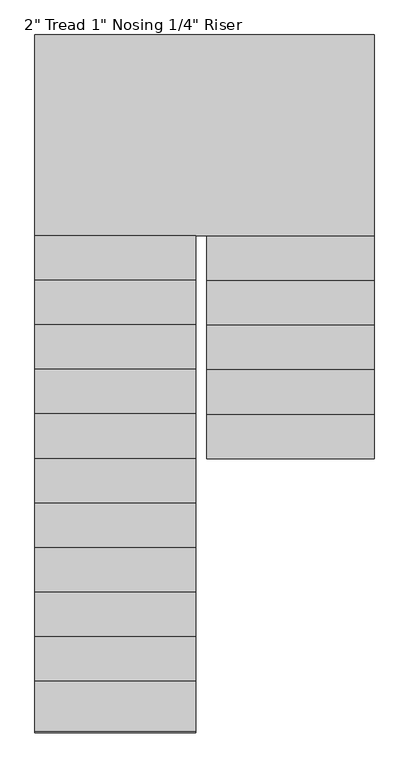
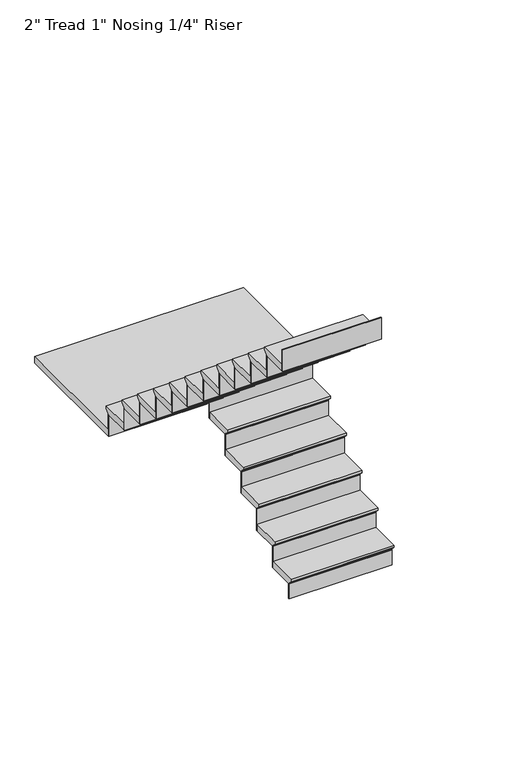
"""IFC4 building model written with IfcOpenShell, lengths in millimetres: stair flight geometry."""

from ifc_helpers import new_model, si_unit, origin, place, context, project, spatial, faceted_brep, source, transform, mapped, element, save


def stair_flight_148faca6(model_context):
    return source(origin(), model_context, "Body", "Brep", [
        faceted_brep([(-3749.597125, 2714.6319226, 39621.8833333), (-3749.597125, 2714.6319226, 39640.9333333), (-4512.2136682, 2714.6319226, 39640.9333333), (-4512.2136682, 2714.6319226, 39621.8833333), (-3749.597125, 2740.0319226, 39596.4833333), (-4512.2136682, 2740.0319226, 39596.4833333), (-3749.597125, 2943.2319226, 39640.9333333), (-4512.2136682, 2943.2319226, 39640.9333333), (-4512.2136682, 2740.0319226, 39590.1333333), (-4512.2136682, 2943.2319226, 39590.1333333), (-3749.597125, 2943.2319226, 39590.1333333), (-3749.597125, 2740.0319226, 39590.1333333)], [[[0, 1, 2, 3]], [[4, 0, 3, 5]], [[2, 1, 6, 7]], [[8, 9, 10, 11]], [[2, 7, 9, 8, 5, 3]], [[8, 11, 4, 5]], [[6, 1, 0, 4, 11, 10]], [[7, 6, 10, 9]]]),
        faceted_brep([(-3749.597125, 2740.0319226, 39590.1333333), (-3749.597125, 2740.0319226, 39471.6), (-3749.597125, 2746.3819226, 39471.6), (-3749.597125, 2746.3819226, 39590.1333333), (-4512.2136682, 2740.0319226, 39590.1333333), (-4512.2136682, 2746.3819226, 39590.1333333), (-4512.2136682, 2746.3819226, 39471.6), (-4512.2136682, 2740.0319226, 39471.6)], [[[0, 1, 2, 3]], [[4, 5, 6, 7]], [[1, 0, 4, 7]], [[2, 1, 7, 6]], [[3, 2, 6, 5]], [[0, 3, 5, 4]]]),
        faceted_brep([(-3749.597125, 2943.2319226, 39759.4666667), (-3749.597125, 2943.2319226, 39590.1333333), (-3749.597125, 2949.5819226, 39590.1333333), (-3749.597125, 2949.5819226, 39759.4666667), (-4512.2136682, 2943.2319226, 39759.4666667), (-4512.2136682, 2949.5819226, 39759.4666667), (-4512.2136682, 2949.5819226, 39590.1333333), (-4512.2136682, 2943.2319226, 39590.1333333)], [[[0, 1, 2, 3]], [[4, 5, 6, 7]], [[1, 0, 4, 7]], [[2, 1, 7, 6]], [[3, 2, 6, 5]], [[0, 3, 5, 4]]]),
        faceted_brep([(-4512.2136682, 2917.8319226, 39810.2666667), (-3749.597125, 2917.8319226, 39810.2666667), (-3749.597125, 3146.4319226, 39810.2666667), (-4512.2136682, 3146.4319226, 39810.2666667), (-4512.2136682, 2943.2319226, 39759.4666667), (-4512.2136682, 3146.4319226, 39759.4666667), (-3749.597125, 3146.4319226, 39759.4666667), (-3749.597125, 2943.2319226, 39759.4666667), (-4512.2136682, 2943.2319226, 39765.8166667), (-4512.2136682, 2917.8319226, 39791.2166667), (-3749.597125, 2943.2319226, 39765.8166667), (-3749.597125, 2917.8319226, 39791.2166667)], [[[0, 1, 2, 3]], [[4, 5, 6, 7]], [[0, 3, 5, 4, 8, 9]], [[4, 7, 10, 8]], [[2, 1, 11, 10, 7, 6]], [[3, 2, 6, 5]], [[11, 1, 0, 9]], [[10, 11, 9, 8]]]),
        faceted_brep([(-3749.597125, 3146.4319226, 39928.8), (-3749.597125, 3146.4319226, 39759.4666667), (-3749.597125, 3152.7819226, 39759.4666667), (-3749.597125, 3152.7819226, 39928.8), (-4512.2136682, 3146.4319226, 39928.8), (-4512.2136682, 3152.7819226, 39928.8), (-4512.2136682, 3152.7819226, 39759.4666667), (-4512.2136682, 3146.4319226, 39759.4666667)], [[[0, 1, 2, 3]], [[4, 5, 6, 7]], [[1, 0, 4, 7]], [[2, 1, 7, 6]], [[3, 2, 6, 5]], [[0, 3, 5, 4]]]),
        faceted_brep([(-4512.2136682, 3121.0319226, 39979.6), (-3749.597125, 3121.0319226, 39979.6), (-3749.597125, 3349.6319226, 39979.6), (-4512.2136682, 3349.6319226, 39979.6), (-4512.2136682, 3146.4319226, 39928.8), (-4512.2136682, 3349.6319226, 39928.8), (-3749.597125, 3349.6319226, 39928.8), (-3749.597125, 3146.4319226, 39928.8), (-4512.2136682, 3146.4319226, 39935.15), (-4512.2136682, 3121.0319226, 39960.55), (-3749.597125, 3146.4319226, 39935.15), (-3749.597125, 3121.0319226, 39960.55)], [[[0, 1, 2, 3]], [[4, 5, 6, 7]], [[0, 3, 5, 4, 8, 9]], [[4, 7, 10, 8]], [[2, 1, 11, 10, 7, 6]], [[3, 2, 6, 5]], [[11, 1, 0, 9]], [[10, 11, 9, 8]]]),
        faceted_brep([(-3749.597125, 3349.6319226, 40098.1333333), (-3749.597125, 3349.6319226, 39928.8), (-3749.597125, 3355.9819226, 39928.8), (-3749.597125, 3355.9819226, 40098.1333333), (-4512.2136682, 3349.6319226, 40098.1333333), (-4512.2136682, 3355.9819226, 40098.1333333), (-4512.2136682, 3355.9819226, 39928.8), (-4512.2136682, 3349.6319226, 39928.8)], [[[0, 1, 2, 3]], [[4, 5, 6, 7]], [[1, 0, 4, 7]], [[2, 1, 7, 6]], [[3, 2, 6, 5]], [[0, 3, 5, 4]]]),
        faceted_brep([(-4512.2136682, 3324.2319226, 40148.9333333), (-3749.597125, 3324.2319226, 40148.9333333), (-3749.597125, 3552.8319226, 40148.9333333), (-4512.2136682, 3552.8319226, 40148.9333333), (-4512.2136682, 3349.6319226, 40098.1333333), (-4512.2136682, 3552.8319226, 40098.1333333), (-3749.597125, 3552.8319226, 40098.1333333), (-3749.597125, 3349.6319226, 40098.1333333), (-4512.2136682, 3349.6319226, 40104.4833333), (-4512.2136682, 3324.2319226, 40129.8833333), (-3749.597125, 3349.6319226, 40104.4833333), (-3749.597125, 3324.2319226, 40129.8833333)], [[[0, 1, 2, 3]], [[4, 5, 6, 7]], [[0, 3, 5, 4, 8, 9]], [[4, 7, 10, 8]], [[2, 1, 11, 10, 7, 6]], [[3, 2, 6, 5]], [[11, 1, 0, 9]], [[10, 11, 9, 8]]]),
        faceted_brep([(-3749.597125, 3552.8319226, 40267.4666667), (-3749.597125, 3552.8319226, 40098.1333333), (-3749.597125, 3559.1819226, 40098.1333333), (-3749.597125, 3559.1819226, 40267.4666667), (-4512.2136682, 3552.8319226, 40267.4666667), (-4512.2136682, 3559.1819226, 40267.4666667), (-4512.2136682, 3559.1819226, 40098.1333333), (-4512.2136682, 3552.8319226, 40098.1333333)], [[[0, 1, 2, 3]], [[4, 5, 6, 7]], [[1, 0, 4, 7]], [[2, 1, 7, 6]], [[3, 2, 6, 5]], [[0, 3, 5, 4]]]),
        faceted_brep([(-4512.2136682, 3527.4319226, 40318.2666667), (-3749.597125, 3527.4319226, 40318.2666667), (-3749.597125, 3756.0319226, 40318.2666667), (-4512.2136682, 3756.0319226, 40318.2666667), (-4512.2136682, 3552.8319226, 40267.4666667), (-4512.2136682, 3756.0319226, 40267.4666667), (-3749.597125, 3756.0319226, 40267.4666667), (-3749.597125, 3552.8319226, 40267.4666667), (-4512.2136682, 3552.8319226, 40273.8166667), (-4512.2136682, 3527.4319226, 40299.2166667), (-3749.597125, 3552.8319226, 40273.8166667), (-3749.597125, 3527.4319226, 40299.2166667)], [[[0, 1, 2, 3]], [[4, 5, 6, 7]], [[0, 3, 5, 4, 8, 9]], [[4, 7, 10, 8]], [[2, 1, 11, 10, 7, 6]], [[3, 2, 6, 5]], [[11, 1, 0, 9]], [[10, 11, 9, 8]]]),
        faceted_brep([(-3749.597125, 3756.0319226, 40436.8), (-3749.597125, 3756.0319226, 40267.4666667), (-3749.597125, 3762.3819226, 40267.4666667), (-3749.597125, 3762.3819226, 40436.8), (-4512.2136682, 3756.0319226, 40436.8), (-4512.2136682, 3762.3819226, 40436.8), (-4512.2136682, 3762.3819226, 40267.4666667), (-4512.2136682, 3756.0319226, 40267.4666667)], [[[0, 1, 2, 3]], [[4, 5, 6, 7]], [[1, 0, 4, 7]], [[2, 1, 7, 6]], [[3, 2, 6, 5]], [[0, 3, 5, 4]]]),
        faceted_brep([(-4563.0136682, 3705.2319226, 40487.6), (-4563.0136682, 3730.6319226, 40487.6), (-3749.597125, 3730.6319226, 40487.6), (-3749.597125, 4645.0319226, 40487.6), (-5295.0246464, 4645.0319226, 40487.6), (-5295.0246464, 3705.2319226, 40487.6), (-4563.0136682, 3730.6319226, 40436.8), (-4563.0136682, 3705.2319226, 40436.8), (-5295.0246464, 3705.2319226, 40436.8), (-5295.0246464, 4645.0319226, 40436.8), (-3749.597125, 4645.0319226, 40436.8), (-3749.597125, 3756.0319226, 40436.8), (-4512.2136682, 3756.0319226, 40436.8), (-4512.2136682, 3730.6319226, 40436.8), (-4512.2136682, 3730.6319226, 40468.55), (-3749.597125, 3730.6319226, 40468.55), (-4512.2136682, 3756.0319226, 40443.15), (-3749.597125, 3756.0319226, 40443.15)], [[[0, 1, 2, 3, 4, 5]], [[6, 7, 8, 9, 10, 11, 12, 13]], [[1, 0, 7, 6]], [[2, 1, 6, 13, 14, 15]], [[13, 12, 16, 14]], [[12, 11, 17, 16]], [[3, 2, 15, 17, 11, 10]], [[4, 3, 10, 9]], [[5, 4, 9, 8]], [[0, 5, 8, 7]], [[17, 15, 14, 16]]]),
        faceted_brep([(-5295.0246464, 3705.2319226, 40606.1333333), (-5295.0246464, 3705.2319226, 40436.8), (-5295.0246464, 3698.8819226, 40436.8), (-5295.0246464, 3698.8819226, 40606.1333333), (-4563.0136682, 3705.2319226, 40606.1333333), (-4563.0136682, 3698.8819226, 40606.1333333), (-4563.0136682, 3698.8819226, 40436.8), (-4563.0136682, 3705.2319226, 40436.8)], [[[0, 1, 2, 3]], [[4, 5, 6, 7]], [[1, 0, 4, 7]], [[2, 1, 7, 6]], [[3, 2, 6, 5]], [[0, 3, 5, 4]]]),
        faceted_brep([(-4563.0136682, 3730.6319226, 40656.9333333), (-5295.0246464, 3730.6319226, 40656.9333333), (-5295.0246464, 3502.0319226, 40656.9333333), (-4563.0136682, 3502.0319226, 40656.9333333), (-4563.0136682, 3705.2319226, 40606.1333333), (-4563.0136682, 3502.0319226, 40606.1333333), (-5295.0246464, 3502.0319226, 40606.1333333), (-5295.0246464, 3705.2319226, 40606.1333333), (-4563.0136682, 3705.2319226, 40612.4833333), (-4563.0136682, 3730.6319226, 40637.8833333), (-5295.0246464, 3705.2319226, 40612.4833333), (-5295.0246464, 3730.6319226, 40637.8833333)], [[[0, 1, 2, 3]], [[4, 5, 6, 7]], [[0, 3, 5, 4, 8, 9]], [[4, 7, 10, 8]], [[2, 1, 11, 10, 7, 6]], [[3, 2, 6, 5]], [[11, 1, 0, 9]], [[10, 11, 9, 8]]]),
        faceted_brep([(-5295.0246464, 3502.0319226, 40775.4666667), (-5295.0246464, 3502.0319226, 40606.1333333), (-5295.0246464, 3495.6819226, 40606.1333333), (-5295.0246464, 3495.6819226, 40775.4666667), (-4563.0136682, 3502.0319226, 40775.4666667), (-4563.0136682, 3495.6819226, 40775.4666667), (-4563.0136682, 3495.6819226, 40606.1333333), (-4563.0136682, 3502.0319226, 40606.1333333)], [[[0, 1, 2, 3]], [[4, 5, 6, 7]], [[1, 0, 4, 7]], [[2, 1, 7, 6]], [[3, 2, 6, 5]], [[0, 3, 5, 4]]]),
        faceted_brep([(-4563.0136682, 3527.4319226, 40826.2666667), (-5295.0246464, 3527.4319226, 40826.2666667), (-5295.0246464, 3298.8319226, 40826.2666667), (-4563.0136682, 3298.8319226, 40826.2666667), (-4563.0136682, 3502.0319226, 40775.4666667), (-4563.0136682, 3298.8319226, 40775.4666667), (-5295.0246464, 3298.8319226, 40775.4666667), (-5295.0246464, 3502.0319226, 40775.4666667), (-4563.0136682, 3502.0319226, 40781.8166667), (-4563.0136682, 3527.4319226, 40807.2166667), (-5295.0246464, 3502.0319226, 40781.8166667), (-5295.0246464, 3527.4319226, 40807.2166667)], [[[0, 1, 2, 3]], [[4, 5, 6, 7]], [[0, 3, 5, 4, 8, 9]], [[4, 7, 10, 8]], [[2, 1, 11, 10, 7, 6]], [[3, 2, 6, 5]], [[11, 1, 0, 9]], [[10, 11, 9, 8]]]),
        faceted_brep([(-5295.0246464, 3298.8319226, 40944.8), (-5295.0246464, 3298.8319226, 40775.4666667), (-5295.0246464, 3292.4819226, 40775.4666667), (-5295.0246464, 3292.4819226, 40944.8), (-4563.0136682, 3298.8319226, 40944.8), (-4563.0136682, 3292.4819226, 40944.8), (-4563.0136682, 3292.4819226, 40775.4666667), (-4563.0136682, 3298.8319226, 40775.4666667)], [[[0, 1, 2, 3]], [[4, 5, 6, 7]], [[1, 0, 4, 7]], [[2, 1, 7, 6]], [[3, 2, 6, 5]], [[0, 3, 5, 4]]]),
        faceted_brep([(-4563.0136682, 3324.2319226, 40995.6), (-5295.0246464, 3324.2319226, 40995.6), (-5295.0246464, 3095.6319226, 40995.6), (-4563.0136682, 3095.6319226, 40995.6), (-4563.0136682, 3298.8319226, 40944.8), (-4563.0136682, 3095.6319226, 40944.8), (-5295.0246464, 3095.6319226, 40944.8), (-5295.0246464, 3298.8319226, 40944.8), (-4563.0136682, 3298.8319226, 40951.15), (-4563.0136682, 3324.2319226, 40976.55), (-5295.0246464, 3298.8319226, 40951.15), (-5295.0246464, 3324.2319226, 40976.55)], [[[0, 1, 2, 3]], [[4, 5, 6, 7]], [[0, 3, 5, 4, 8, 9]], [[4, 7, 10, 8]], [[2, 1, 11, 10, 7, 6]], [[3, 2, 6, 5]], [[11, 1, 0, 9]], [[10, 11, 9, 8]]]),
        faceted_brep([(-5295.0246464, 3095.6319226, 41114.1333333), (-5295.0246464, 3095.6319226, 40944.8), (-5295.0246464, 3089.2819226, 40944.8), (-5295.0246464, 3089.2819226, 41114.1333333), (-4563.0136682, 3095.6319226, 41114.1333333), (-4563.0136682, 3089.2819226, 41114.1333333), (-4563.0136682, 3089.2819226, 40944.8), (-4563.0136682, 3095.6319226, 40944.8)], [[[0, 1, 2, 3]], [[4, 5, 6, 7]], [[1, 0, 4, 7]], [[2, 1, 7, 6]], [[3, 2, 6, 5]], [[0, 3, 5, 4]]]),
        faceted_brep([(-4563.0136682, 3121.0319226, 41164.9333333), (-5295.0246464, 3121.0319226, 41164.9333333), (-5295.0246464, 2892.4319226, 41164.9333333), (-4563.0136682, 2892.4319226, 41164.9333333), (-4563.0136682, 3095.6319226, 41114.1333333), (-4563.0136682, 2892.4319226, 41114.1333333), (-5295.0246464, 2892.4319226, 41114.1333333), (-5295.0246464, 3095.6319226, 41114.1333333), (-4563.0136682, 3095.6319226, 41120.4833333), (-4563.0136682, 3121.0319226, 41145.8833333), (-5295.0246464, 3095.6319226, 41120.4833333), (-5295.0246464, 3121.0319226, 41145.8833333)], [[[0, 1, 2, 3]], [[4, 5, 6, 7]], [[0, 3, 5, 4, 8, 9]], [[4, 7, 10, 8]], [[2, 1, 11, 10, 7, 6]], [[3, 2, 6, 5]], [[11, 1, 0, 9]], [[10, 11, 9, 8]]]),
        faceted_brep([(-5295.0246464, 2892.4319226, 41283.4666667), (-5295.0246464, 2892.4319226, 41114.1333333), (-5295.0246464, 2886.0819226, 41114.1333333), (-5295.0246464, 2886.0819226, 41283.4666667), (-4563.0136682, 2892.4319226, 41283.4666667), (-4563.0136682, 2886.0819226, 41283.4666667), (-4563.0136682, 2886.0819226, 41114.1333333), (-4563.0136682, 2892.4319226, 41114.1333333)], [[[0, 1, 2, 3]], [[4, 5, 6, 7]], [[1, 0, 4, 7]], [[2, 1, 7, 6]], [[3, 2, 6, 5]], [[0, 3, 5, 4]]]),
        faceted_brep([(-4563.0136682, 2917.8319226, 41334.2666667), (-5295.0246464, 2917.8319226, 41334.2666667), (-5295.0246464, 2689.2319226, 41334.2666667), (-4563.0136682, 2689.2319226, 41334.2666667), (-4563.0136682, 2892.4319226, 41283.4666667), (-4563.0136682, 2689.2319226, 41283.4666667), (-5295.0246464, 2689.2319226, 41283.4666667), (-5295.0246464, 2892.4319226, 41283.4666667), (-4563.0136682, 2892.4319226, 41289.8166667), (-4563.0136682, 2917.8319226, 41315.2166667), (-5295.0246464, 2892.4319226, 41289.8166667), (-5295.0246464, 2917.8319226, 41315.2166667)], [[[0, 1, 2, 3]], [[4, 5, 6, 7]], [[0, 3, 5, 4, 8, 9]], [[4, 7, 10, 8]], [[2, 1, 11, 10, 7, 6]], [[3, 2, 6, 5]], [[11, 1, 0, 9]], [[10, 11, 9, 8]]]),
        faceted_brep([(-5295.0246464, 2689.2319226, 41452.8), (-5295.0246464, 2689.2319226, 41283.4666667), (-5295.0246464, 2682.8819226, 41283.4666667), (-5295.0246464, 2682.8819226, 41452.8), (-4563.0136682, 2689.2319226, 41452.8), (-4563.0136682, 2682.8819226, 41452.8), (-4563.0136682, 2682.8819226, 41283.4666667), (-4563.0136682, 2689.2319226, 41283.4666667)], [[[0, 1, 2, 3]], [[4, 5, 6, 7]], [[1, 0, 4, 7]], [[2, 1, 7, 6]], [[3, 2, 6, 5]], [[0, 3, 5, 4]]]),
        faceted_brep([(-4563.0136682, 2714.6319226, 41503.6), (-5295.0246464, 2714.6319226, 41503.6), (-5295.0246464, 2486.0319226, 41503.6), (-4563.0136682, 2486.0319226, 41503.6), (-4563.0136682, 2689.2319226, 41452.8), (-4563.0136682, 2486.0319226, 41452.8), (-5295.0246464, 2486.0319226, 41452.8), (-5295.0246464, 2689.2319226, 41452.8), (-4563.0136682, 2689.2319226, 41459.15), (-4563.0136682, 2714.6319226, 41484.55), (-5295.0246464, 2689.2319226, 41459.15), (-5295.0246464, 2714.6319226, 41484.55)], [[[0, 1, 2, 3]], [[4, 5, 6, 7]], [[0, 3, 5, 4, 8, 9]], [[4, 7, 10, 8]], [[2, 1, 11, 10, 7, 6]], [[3, 2, 6, 5]], [[11, 1, 0, 9]], [[10, 11, 9, 8]]]),
        faceted_brep([(-5295.0246464, 2486.0319226, 41622.1333333), (-5295.0246464, 2486.0319226, 41452.8), (-5295.0246464, 2479.6819226, 41452.8), (-5295.0246464, 2479.6819226, 41622.1333333), (-4563.0136682, 2486.0319226, 41622.1333333), (-4563.0136682, 2479.6819226, 41622.1333333), (-4563.0136682, 2479.6819226, 41452.8), (-4563.0136682, 2486.0319226, 41452.8)], [[[0, 1, 2, 3]], [[4, 5, 6, 7]], [[1, 0, 4, 7]], [[2, 1, 7, 6]], [[3, 2, 6, 5]], [[0, 3, 5, 4]]]),
        faceted_brep([(-4563.0136682, 2511.4319226, 41672.9333333), (-5295.0246464, 2511.4319226, 41672.9333333), (-5295.0246464, 2282.8319226, 41672.9333333), (-4563.0136682, 2282.8319226, 41672.9333333), (-4563.0136682, 2486.0319226, 41622.1333333), (-4563.0136682, 2282.8319226, 41622.1333333), (-5295.0246464, 2282.8319226, 41622.1333333), (-5295.0246464, 2486.0319226, 41622.1333333), (-4563.0136682, 2486.0319226, 41628.4833333), (-4563.0136682, 2511.4319226, 41653.8833333), (-5295.0246464, 2486.0319226, 41628.4833333), (-5295.0246464, 2511.4319226, 41653.8833333)], [[[0, 1, 2, 3]], [[4, 5, 6, 7]], [[0, 3, 5, 4, 8, 9]], [[4, 7, 10, 8]], [[2, 1, 11, 10, 7, 6]], [[3, 2, 6, 5]], [[11, 1, 0, 9]], [[10, 11, 9, 8]]]),
        faceted_brep([(-5295.0246464, 2282.8319226, 41791.4666667), (-5295.0246464, 2282.8319226, 41622.1333333), (-5295.0246464, 2276.4819226, 41622.1333333), (-5295.0246464, 2276.4819226, 41791.4666667), (-4563.0136682, 2282.8319226, 41791.4666667), (-4563.0136682, 2276.4819226, 41791.4666667), (-4563.0136682, 2276.4819226, 41622.1333333), (-4563.0136682, 2282.8319226, 41622.1333333)], [[[0, 1, 2, 3]], [[4, 5, 6, 7]], [[1, 0, 4, 7]], [[2, 1, 7, 6]], [[3, 2, 6, 5]], [[0, 3, 5, 4]]]),
        faceted_brep([(-4563.0136682, 2308.2319226, 41842.2666667), (-5295.0246464, 2308.2319226, 41842.2666667), (-5295.0246464, 2079.6319226, 41842.2666667), (-4563.0136682, 2079.6319226, 41842.2666667), (-4563.0136682, 2282.8319226, 41791.4666667), (-4563.0136682, 2079.6319226, 41791.4666667), (-5295.0246464, 2079.6319226, 41791.4666667), (-5295.0246464, 2282.8319226, 41791.4666667), (-4563.0136682, 2282.8319226, 41797.8166667), (-4563.0136682, 2308.2319226, 41823.2166667), (-5295.0246464, 2282.8319226, 41797.8166667), (-5295.0246464, 2308.2319226, 41823.2166667)], [[[0, 1, 2, 3]], [[4, 5, 6, 7]], [[0, 3, 5, 4, 8, 9]], [[4, 7, 10, 8]], [[2, 1, 11, 10, 7, 6]], [[3, 2, 6, 5]], [[11, 1, 0, 9]], [[10, 11, 9, 8]]]),
        faceted_brep([(-5295.0246464, 2079.6319226, 41960.8), (-5295.0246464, 2079.6319226, 41791.4666667), (-5295.0246464, 2073.2819226, 41791.4666667), (-5295.0246464, 2073.2819226, 41960.8), (-4563.0136682, 2079.6319226, 41960.8), (-4563.0136682, 2073.2819226, 41960.8), (-4563.0136682, 2073.2819226, 41791.4666667), (-4563.0136682, 2079.6319226, 41791.4666667)], [[[0, 1, 2, 3]], [[4, 5, 6, 7]], [[1, 0, 4, 7]], [[2, 1, 7, 6]], [[3, 2, 6, 5]], [[0, 3, 5, 4]]]),
        faceted_brep([(-4563.0136682, 2105.0319226, 42011.6), (-5295.0246464, 2105.0319226, 42011.6), (-5295.0246464, 1876.4319226, 42011.6), (-4563.0136682, 1876.4319226, 42011.6), (-4563.0136682, 2079.6319226, 41960.8), (-4563.0136682, 1876.4319226, 41960.8), (-5295.0246464, 1876.4319226, 41960.8), (-5295.0246464, 2079.6319226, 41960.8), (-4563.0136682, 2079.6319226, 41967.15), (-4563.0136682, 2105.0319226, 41992.55), (-5295.0246464, 2079.6319226, 41967.15), (-5295.0246464, 2105.0319226, 41992.55)], [[[0, 1, 2, 3]], [[4, 5, 6, 7]], [[0, 3, 5, 4, 8, 9]], [[4, 7, 10, 8]], [[2, 1, 11, 10, 7, 6]], [[3, 2, 6, 5]], [[11, 1, 0, 9]], [[10, 11, 9, 8]]]),
        faceted_brep([(-5295.0246464, 1876.4319226, 42130.1333333), (-5295.0246464, 1876.4319226, 41960.8), (-5295.0246464, 1870.0819226, 41960.8), (-5295.0246464, 1870.0819226, 42130.1333333), (-4563.0136682, 1876.4319226, 42130.1333333), (-4563.0136682, 1870.0819226, 42130.1333333), (-4563.0136682, 1870.0819226, 41960.8), (-4563.0136682, 1876.4319226, 41960.8)], [[[0, 1, 2, 3]], [[4, 5, 6, 7]], [[1, 0, 4, 7]], [[2, 1, 7, 6]], [[3, 2, 6, 5]], [[0, 3, 5, 4]]]),
        faceted_brep([(-4563.0136682, 1901.8319226, 42180.9333333), (-5295.0246464, 1901.8319226, 42180.9333333), (-5295.0246464, 1673.2319226, 42180.9333333), (-4563.0136682, 1673.2319226, 42180.9333333), (-4563.0136682, 1876.4319226, 42130.1333333), (-4563.0136682, 1673.2319226, 42130.1333333), (-5295.0246464, 1673.2319226, 42130.1333333), (-5295.0246464, 1876.4319226, 42130.1333333), (-4563.0136682, 1876.4319226, 42136.4833333), (-4563.0136682, 1901.8319226, 42161.8833333), (-5295.0246464, 1876.4319226, 42136.4833333), (-5295.0246464, 1901.8319226, 42161.8833333)], [[[0, 1, 2, 3]], [[4, 5, 6, 7]], [[0, 3, 5, 4, 8, 9]], [[4, 7, 10, 8]], [[2, 1, 11, 10, 7, 6]], [[3, 2, 6, 5]], [[11, 1, 0, 9]], [[10, 11, 9, 8]]]),
        faceted_brep([(-5295.0246464, 1673.2319226, 42299.4666667), (-5295.0246464, 1673.2319226, 42130.1333333), (-5295.0246464, 1666.8819226, 42130.1333333), (-5295.0246464, 1666.8819226, 42299.4666667), (-4563.0136682, 1673.2319226, 42299.4666667), (-4563.0136682, 1666.8819226, 42299.4666667), (-4563.0136682, 1666.8819226, 42130.1333333), (-4563.0136682, 1673.2319226, 42130.1333333)], [[[0, 1, 2, 3]], [[4, 5, 6, 7]], [[1, 0, 4, 7]], [[2, 1, 7, 6]], [[3, 2, 6, 5]], [[0, 3, 5, 4]]]),
        faceted_brep([(-4563.0136682, 1698.6319226, 42350.2666667), (-5295.0246464, 1698.6319226, 42350.2666667), (-5295.0246464, 1470.0319226, 42350.2666667), (-4563.0136682, 1470.0319226, 42350.2666667), (-4563.0136682, 1673.2319226, 42299.4666667), (-4563.0136682, 1470.0319226, 42299.4666667), (-5295.0246464, 1470.0319226, 42299.4666667), (-5295.0246464, 1673.2319226, 42299.4666667), (-4563.0136682, 1673.2319226, 42305.8166667), (-4563.0136682, 1698.6319226, 42331.2166667), (-5295.0246464, 1673.2319226, 42305.8166667), (-5295.0246464, 1698.6319226, 42331.2166667)], [[[0, 1, 2, 3]], [[4, 5, 6, 7]], [[0, 3, 5, 4, 8, 9]], [[4, 7, 10, 8]], [[2, 1, 11, 10, 7, 6]], [[3, 2, 6, 5]], [[11, 1, 0, 9]], [[10, 11, 9, 8]]]),
        faceted_brep([(-5295.0246464, 1470.0319226, 42468.8), (-5295.0246464, 1470.0319226, 42299.4666667), (-5295.0246464, 1463.6819226, 42299.4666667), (-5295.0246464, 1463.6819226, 42468.8), (-4563.0136682, 1470.0319226, 42468.8), (-4563.0136682, 1463.6819226, 42468.8), (-4563.0136682, 1463.6819226, 42299.4666667), (-4563.0136682, 1470.0319226, 42299.4666667)], [[[0, 1, 2, 3]], [[4, 5, 6, 7]], [[1, 0, 4, 7]], [[2, 1, 7, 6]], [[3, 2, 6, 5]], [[0, 3, 5, 4]]]),
    ])


if __name__ == "__main__":
    model = new_model("IFC4")
    model_context = context("Model", 3, world=origin())
    ifc_project = project(units=[si_unit("LENGTHUNIT", "METRE", prefix="MILLI")], contexts=[model_context])
    site = spatial("IfcSite", under=ifc_project)
    building = spatial("IfcBuilding", under=site)
    placement = place(None, origin())
    stair_flight_shape = stair_flight_148faca6(model_context)
    element("IfcStairFlight", 1, ObjectType="2\" Tread 1\" Nosing 1/4\" Riser", at=placement, inside=building, context=model_context, shape_type="MappedRepresentation", body=[
        mapped(stair_flight_shape, transform((0.0, 0.0, 0.0), x_axis=(1.0, 0.0, 0.0), y_axis=(0.0, 1.0, 0.0), z_axis=(0.0, 0.0, 1.0))),
    ])
    save(model, "model.ifc")
